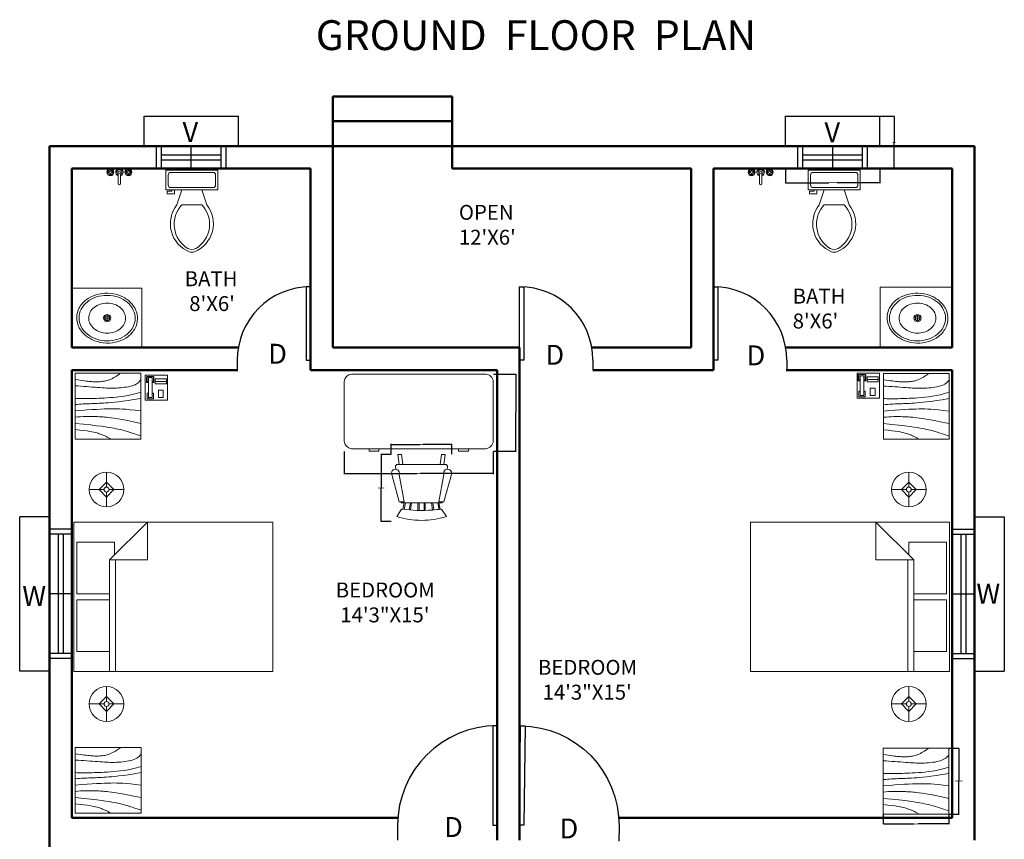
# Model space of a CAD drawing. Units: inches. Extents: x -8 to 1354, y -679 to 94.
# Tile 3 of 6: x -8 to 388, y -248 to 81. Entities that reach past the tile are written whole.
import ezdxf

# ---------------------------------------------------------------- set-up
doc = ezdxf.new("R2010")
doc.units = ezdxf.units.IN
doc.header["$MEASUREMENT"] = 0
for name, color, linetype, lineweight in [('A-ANNO-DIMS', 2, 'Continuous', 18), ('A-ANNO-TEXT', 7, 'Continuous', 25), ('A-AREA-IDEN', 7, 'Continuous', 25), ('A-DOOR', 3, 'Continuous', 25), ('A-FLOR-FIXT', 8, 'Continuous', 18), ('A-FURN', 8, 'Continuous', 18), ('A-GLAZ', 4, 'Continuous', 25), ('A-WALL', 1, 'Continuous', 50)]:
    doc.layers.add(name, color=color, linetype=linetype, lineweight=lineweight)
doc.styles.get("Standard").update_dxf_attribs({"font": 'arial.ttf'})
doc.dimstyles.get("Standard").update_dxf_attribs({"dimtxt": 0.18, "dimasz": 0.18, "dimexe": 0.18, "dimexo": 0.0625, "dimgap": 0.09, "dimtad": 0, "dimtih": 1, "dimtoh": 1, "dimdec": 1, "dimzin": 0, "dimdsep": 46, "dimlunit": 4, "dimtxsty": 'Standard', "dimcen": 0.09, "dimclrd": 2, "dimclre": 3, "dimclrt": 6, "dimadec": 0, "dimazin": 0, "dimtfac": 1, "dimtdec": 1, "dimtofl": 0, "dimtmove": 0, "dimatfit": 3, "dimfxl": 1, "dimtfill": 2, "dimtfillclr": 4, "dimtolj": 1, "dimtzin": 0, "dimarcsym": 0})

# ---------------------------------------------------------------- blocks, each defined once
blk = doc.blocks.new('*U6')
for p, q in [((0, 0), (0, -6)), ((-40, 0), (-40, -6))]:
    blk.add_line(p, q)
blk.add_lwpolyline([(0, 0), (0, 40), (-1.75, 40), (-1.75, 0)], close=True)
blk.add_arc((0, 0), 40, 90, 180)
blk = doc.blocks.new('*U4')
for p, q in [((0, 0), (0, -100)), ((750, 0), (750, -100))]:
    blk.add_line(p, q)
blk.add_lwpolyline([(0, 0), (0, 750), (43.75, 750), (43.75, 0)], close=True)
blk.add_arc((0, 0), 750, 0, 90)
blk = doc.blocks.new('*U7')
for p, q in [((-750, 0), (-750, -100)), ((0, 0), (0, -100))]:
    blk.add_line(p, q)
blk.add_lwpolyline([(0, 0), (0, 750), (-43.75, 750), (-43.75, 0)], close=True)
blk.add_arc((0, 0), 750, 90, 180)
blk = doc.blocks.new('Bed - Queen')
for p, q in [((0, -80.00003), (0, 0)), ((0, 0), (59.99999, 0)), ((59.99999, 0), (59.99999, -80.00003)), ((7.99999, -1.2), (28.79998, -1.2)), ((7.99999, -14.4), (7.99999, -1.2)), ((28.79998, -1.2), (28.79998, -14.4)), ((31.19999, -1.2), (51.99999, -1.2)), ((31.19999, -14.4), (31.19999, -1.2)), ((51.99999, -1.2), (51.99999, -16.4)), ((0, -14.4), (44.8, -14.4)), ((59.99999, -29.6), (44.8, -14.4)), ((44.8, -14.4), (44.8, -29.6)), ((44.8, -16.8), (0, -16.8)), ((51.99999, -16.4), (46.79936, -16.4)), ((44.8, -29.6), (59.99999, -29.6)), ((59.99999, -80.00003), (0, -80.00003))]:
    blk.add_line(p, q)
blk = doc.blocks.new('Chair - Rocking')
for p, q in [((-8, -4.5), (-10, -1.5)), ((8, -4.5), (10, -1.5)), ((-9, -7.5), (-12, -18.49999)), ((-7, -7.5), (-9, -7.5)), ((-9, -18.49999), (-7, -7.5)), ((-8.23428, -6.99939), (-8.3093, -7.47958)), ((-8.23041, -7), (8.23915, -7)), ((-7.5, -4.5), (-7, -7)), ((-6.5, -7), (-7.02225, -4.43)), ((-4.5, -7), (-4.96674, -4.19951)), ((-4, -7), (-4.40532, -4.16272)), ((-1.5, -4.05012), (-1.5, -7)), ((-1, -7), (-1, -4.05012)), ((1, -7), (1, -4.04655)), ((1.5, -4.05012), (1.5, -7)), ((4, -7), (4.40187, -4.18694)), ((4.5, -7), (4.96761, -4.19437)), ((6.5, -7), (7, -4.4057)), ((7.5, -4.5), (7, -7)), ((7, -7.5), (9, -7.5)), ((9, -18.49999), (7, -7.5)), ((8.31071, -7.48854), (8.23449, -7.00073)), ((9, -7.5), (12, -18.49999)), ((-10.36644, -20.64523), (-10.5, -21.49999)), ((-9, -22.49999), (-9.5, -26.49999)), ((0, -22.49999), (-9.5, -22.49999)), ((-8, -26.49999), (-7.5, -22.49999)), ((0, -22.49999), (9.5, -22.49999)), ((8, -26.49999), (7.5, -22.49999)), ((9, -22.49999), (9.5, -26.49999)), ((10.5, -21.49999), (10.3575, -20.58798)), ((-9.5, -26.49999), (-8, -26.49999)), ((9.5, -26.49999), (8, -26.49999))]:
    blk.add_line(p, q)
for centre, radius, start, end in [((0, -34.08333), 34.08333, 72.93847, 107.0615), ((0, -68.25004), 64.25, 93.92211, 97.15267), ((0, -68.25004), 64.25, 82.84733, 93.92211), ((-10.5, -18.99999), 1.58114, 161.5651, 18.43495), ((10.5, -18.99999), 1.58114, 161.5651, 18.43495), ((-9.5, -21.49999), 1, 180, 270), ((9.5, -21.49999), 1, 270, 0)]:
    blk.add_arc(centre, radius, start, end)
blk = doc.blocks.new('Desk - 30 x 60 in.')
for p, q in [((-26.999995, 0), (26.999995, 0)), ((-29.999995, -27), (-29.999995, -3)), ((29.999995, -3), (29.999995, -27)), ((26.999995, -30), (-26.999995, -30)), ((-20.000005, -30), (-20.000005, -31)), ((-20.000005, -31), (-16.000005, -31)), ((-16.000005, -31), (-16.000005, -30)), ((15.999995, -31), (15.999995, -30)), ((19.999995, -31), (15.999995, -31)), ((19.999995, -30), (19.999995, -31))]:
    blk.add_line(p, q)
for centre, start, end in [((-26.499995, -3.5), 98.1301, 171.8699), ((26.499995, -3.5), 8.130102, 81.8699), ((-26.499995, -26.5), 188.1301, 261.8699), ((26.499995, -26.5), 278.1301, 351.8699)]:
    blk.add_arc(centre, 3.535534, start, end)
blk = doc.blocks.new('Lamp - Table')
for p, q in [((0, 7), (0, 1)), ((-1, 0), (-7, 0)), ((0, 3), (-3, 0)), ((-3, 0), (0, -3)), ((3, 0), (0, 3)), ((0, -3), (3, 0)), ((1, 0), (7, 0)), ((0, -1), (0, -7))]:
    blk.add_line(p, q)
for radius in [7, 1]:
    blk.add_circle((0, 0), radius)
blk = doc.blocks.new('Phone - Desk')
for p, q in [((-4.5, -5), (-4.5, 5)), ((-4.5, 5), (4.5, 5)), ((-4, 4.5), (-4, 2)), ((-3.75, 4.5), (-3.75, 2.25)), ((-1.25, 4.5), (-3.75, 4.5)), ((-3.25, 4), (-3.25, -4)), ((-3.25, 4), (-1.75, 4)), ((-1.75, -4), (-1.75, 4)), ((-1.25, 2.25), (-1.25, 4.5)), ((-1, 2), (-1, 4.5)), ((4.5, 5), (4.5, -5)), ((-4, 2), (-3.25, 2)), ((-3.75, 2.25), (-3.25, 2.25)), ((-1.75, 2.25), (-1.25, 2.25)), ((-1.75, 2), (-1, 2)), ((4, 3.5), (-0.5, 3.5)), ((-0.5, 3.5), (-0.5, 1.5)), ((-0.5, 2.5), (4, 2.5)), ((-0.5, 1.5), (4, 1.5)), ((4, 1.5), (4, 3.5)), ((-3.75, -2.25), (-3.25, -2.25)), ((-3.75, -4.5), (-3.75, -2.25)), ((-1.75, -2.25), (-1.25, -2.25)), ((-1.25, -2.25), (-1.25, -4.5)), ((2.75, -1), (0.75, -1)), ((0.75, -1), (0.75, -4)), ((2.75, -4), (2.75, -1)), ((4.5, -5), (-4.5, -5)), ((-1.25, -4.5), (-3.75, -4.5)), ((-3.25, -4), (-1.75, -4)), ((0.75, -4), (2.75, -4))]:
    blk.add_line(p, q)
blk = doc.blocks.new('Table - Square Woodgrain 42 x 42 in.')
blk.add_line((0, -42), (42, -42))
for points in [[(0, -4), (1.704, -4.2172), (3.2358, -4.4188), (4.615, -4.604), (5.8615, -4.7721), (6.9951, -4.9224), (8.0357, -5.0541), (9.0031, -5.1667), (9.9171, -5.2594), (10.7951, -5.3316), (11.6445, -5.3836), (12.4702, -5.4157), (13.277, -5.4283), (14.0698, -5.4217), (14.8535, -5.3964), (15.6331, -5.3526), (16.4133, -5.2908), (17.1986, -5.2103), (17.9913, -5.1062), (18.793, -4.9727), (19.6056, -4.8038), (20.4307, -4.5937), (21.2701, -4.3365), (22.1256, -4.0262), (22.9989, -3.6571), (23.888, -3.2272), (24.7756, -2.7516), (25.6408, -2.2491), (26.4624, -1.7387), (27.2195, -1.2395), (27.891, -0.7703), (28.456, -0.3501), (28.8934, 0.002)], [(0, -42), (0, 0), (42, 0), (42, -42)], [(0, -8), (1.8203, -8.1001), (3.6741, -8.2149), (5.5411, -8.3408), (7.4011, -8.4741), (9.2339, -8.6112), (11.0193, -8.7484), (12.7371, -8.8821), (14.3671, -9.0086), (15.8954, -9.1246), (17.3337, -9.2278), (18.6997, -9.3159), (20.0116, -9.387), (21.2871, -9.4389), (22.5442, -9.4696), (23.8008, -9.477), (25.0749, -9.459), (26.3791, -9.4137), (27.7049, -9.3403), (29.0383, -9.2382), (30.3655, -9.1068), (31.6728, -8.9455), (32.9461, -8.7535), (34.1717, -8.5304), (35.3358, -8.2756), (36.4268, -7.9863), (37.443, -7.6521), (38.3849, -7.2603), (39.253, -6.7986), (40.048, -6.2542), (40.7705, -5.6147), (41.421, -4.8674), (42, -4)], [(42, -12), (39.1784, -12.8621), (36.4519, -13.5654), (33.8246, -14.1294), (31.3004, -14.5731), (28.8832, -14.9161), (26.577, -15.1775), (24.3858, -15.3768), (22.3136, -15.5332), (20.3622, -15.6632), (18.5254, -15.7718), (16.7947, -15.8612), (15.1618, -15.9338), (13.6183, -15.9916), (12.1558, -16.0369), (10.7659, -16.0718), (9.4403, -16.0987), (8.1703, -16.1191), (6.9461, -16.1325), (5.7577, -16.1377), (4.595, -16.1335), (3.4479, -16.1188), (2.3064, -16.0924), (1.1604, -16.0532), (0, -16)], [(42, -16), (37.6529, -16.7365), (33.8802, -17.329), (30.6179, -17.7961), (27.8015, -18.1561), (25.3668, -18.4275), (23.2497, -18.6288), (21.3859, -18.7785), (19.7111, -18.8949), (18.1693, -18.9939), (16.7375, -19.0795), (15.401, -19.1534), (14.1449, -19.217), (12.9544, -19.2717), (11.8148, -19.3191), (10.7113, -19.3606), (9.6291, -19.3976), (8.5534, -19.4323), (7.47, -19.4689), (6.3643, -19.5122), (5.222, -19.5672), (4.0288, -19.6386), (2.7703, -19.7313), (1.4321, -19.8501), (0, -20)], [(0, -24), (3.9243, -23.6805), (7.4766, -23.4138), (10.6891, -23.1954), (13.5943, -23.0205), (16.2247, -22.8847), (18.6125, -22.7832), (20.7903, -22.7116), (22.7903, -22.6651), (24.6563, -22.642), (26.4764, -22.6507), (28.35, -22.7024), (30.3766, -22.8084), (32.6555, -22.98), (35.2861, -23.2283), (38.3678, -23.5645), (42, -24)], [(42, -32), (37.392, -31.017), (33.4585, -30.2231), (30.1291, -29.5949), (27.3334, -29.109), (25.0009, -28.742), (23.0612, -28.4707), (21.4439, -28.2716), (20.0786, -28.1215), (18.8998, -28.0002), (17.8609, -27.9014), (16.9206, -27.8219), (16.0371, -27.7588), (15.1691, -27.709), (14.2748, -27.6693), (13.3128, -27.6368), (12.2415, -27.6083), (11.0295, -27.5824), (9.6867, -27.5643), (8.233, -27.5608), (6.6884, -27.5787), (5.0728, -27.6248), (3.4062, -27.7058), (1.7086, -27.8286), (0, -28)], [(0, -32), (5.4026, -32.5358), (9.9494, -33.019), (13.7424, -33.4553), (16.8834, -33.8505), (19.4743, -34.2106), (21.6171, -34.5413), (23.4136, -34.8486), (24.9657, -35.1382), (26.3614, -35.4156), (27.6332, -35.6841), (28.7995, -35.9467), (29.8788, -36.2064), (30.8897, -36.4661), (31.8507, -36.7288), (32.7802, -36.9973), (33.6968, -37.2747), (34.6175, -37.5635), (35.5531, -37.8651), (36.5128, -38.1805), (37.506, -38.5108), (38.5421, -38.8568), (39.6302, -39.2197), (40.7797, -39.6004), (42, -40)], [(0, -36), (3.0098, -36.2857), (5.5354, -36.5643), (7.6368, -36.8359), (9.374, -37.1009), (10.807, -37.3597), (11.9957, -37.6126), (13.0002, -37.8599), (13.8804, -38.102), (14.6874, -38.3393), (15.4365, -38.5729), (16.1338, -38.8041), (16.7858, -39.0341), (17.3987, -39.264), (17.9787, -39.4952), (18.5322, -39.7288), (19.0655, -39.9662), (19.5832, -40.2081), (20.0842, -40.4544), (20.5657, -40.7046), (21.0249, -40.9581), (21.459, -41.2144), (21.8653, -41.4731), (22.2409, -41.7335), (22.5831, -41.9951)]]:
    blk.add_lwpolyline(points)
blk = doc.blocks.new('Sink - Oval top')
for p, q in [((-1, 0), (1, 0)), ((0, 1), (0, -1))]:
    blk.add_line(p, q)
for points in [[(-12.23, 0.39, 0.117634), (-11.46, -3.36, 0.104469), (-8.88, -6.8, 0.090016), (-5.08, -9.07, 0.08192), (-0.32, -10.02, 0.08192), (4.49, -9.38, 0.090016), (8.42, -7.36, 0.104469), (11.22, -4.09, 0.117634), (12.23, -0.39, 0.117634), (11.46, 3.36, 0.104469), (8.88, 6.8, 0.090016), (5.08, 9.07, 0.08192), (0.32, 10.02, 0.08192), (-4.49, 9.38, 0.090016), (-8.42, 7.36, 0.104469), (-11.22, 4.09, 0.117634)], [(-11.29, 0.16, 0.118622), (-10.52, -3.25, 0.104678), (-8.07, -6.36, 0.089562), (-4.54, -8.37, 0.081185), (-0.13, -9.15, 0.081185), (4.3, -8.49, 0.089562), (7.89, -6.58, 0.104678), (10.42, -3.55, 0.118622), (11.29, -0.16, 0.118622), (10.52, 3.25, 0.104678), (8.07, 6.36, 0.089562), (4.54, 8.37, 0.081185), (0.13, 9.15, 0.081185), (-4.3, 8.49, 0.089562), (-7.89, 6.58, 0.104678), (-10.42, 3.55, 0.118622)], [(-7.42, 0.08, 0.118283), (-6.91, -2.17, 0.104607), (-5.29, -4.21, 0.089718), (-2.97, -5.53, 0.081436), (-0.07, -6.04, 0.081436), (2.84, -5.59, 0.089718), (5.2, -4.33, 0.104607), (6.86, -2.32, 0.118283), (7.42, -0.08, 0.118283), (6.91, 2.17, 0.104607), (5.29, 4.21, 0.089718), (2.97, 5.53, 0.081436), (0.07, 6.04, 0.081436), (-2.84, 5.59, 0.089718), (-5.2, 4.33, 0.104607), (-6.86, 2.32, 0.118283)]]:
    blk.add_lwpolyline(points, format="xyb", close=True)
for radius in [1.5, 1]:
    blk.add_circle((0, 0), radius)
blk = doc.blocks.new('Toilet - top')
for p, q in [((9.5, -6), (9.5, -2)), ((-10, -8.5), (-8, -8.5)), ((-10, -9.5), (-10, -8.5)), ((-7, -9.5), (-10, -9.5)), ((-8, -8.5), (-8, -8)), ((-7, -8), (-7, -9.5)), ((-4, -8), (-6, -14)), ((4, -8), (6, -14)), ((4, -14), (-4, -14))]:
    blk.add_line(p, q)
blk.add_lwpolyline([(10.5, -8), (10.5, 0), (-10.5, 0), (-10.5, -8)], close=True)
for points in [[(-9.5, -2), (-9.5, -6)], [(8.5, -1), (-8.5, -1)], [(-8.5, -7), (8.5, -7)]]:
    blk.add_lwpolyline(points)
for centre, radius, start, end in [((-8.62, -1.88), 0.884, 81.8699, 188.1301), ((8.62, -1.88), 0.884, 351.8699, 98.1301), ((-8.62, -6.12), 0.884, 171.8699, 278.1301), ((8.62, -6.12), 0.884, 261.8699, 8.1301), ((3.52, -21.58), 12.17, 141.4691, 247.9714), ((4.2, -21.82), 11.33, 136.3677, 238.9468), ((-3.52, -21.58), 12.17, 292.0284, 38.5307), ((-4.2, -21.82), 11.33, 301.053, 43.6321), ((0, -27.88), 4, 245.7318, 294.2682), ((0, -29), 4, 254.8605, 285.1395)]:
    blk.add_arc(centre, radius, start, end)
blk = doc.blocks.new('Faucet - Bathroom top')
for p, q in [((-4.107, 0.125), (-4.375, 0.125)), ((-3.75, 0.4788), (-3.75, 0.75)), ((-3.5, 0.482), (-3.5, 0.75)), ((-3.1461, 0.125), (-2.875, 0.125)), ((3.143, 0.125), (2.875, 0.125)), ((3.5, 0.4788), (3.5, 0.75)), ((3.75, 0.482), (3.75, 0.75)), ((4.1039, 0.125), (4.375, 0.125)), ((-4.1039, -0.125), (-4.375, -0.125)), ((-3.75, -0.4821), (-3.75, -0.75)), ((-3.5, -0.4789), (-3.5, -0.75)), ((-3.143, -0.125), (-2.875, -0.125)), ((-0.5, -0.8639), (-0.5, -4.5)), ((0.5, -4.5), (0.5, -0.8631)), ((3.1461, -0.125), (2.875, -0.125)), ((3.5, -0.4821), (3.5, -0.75)), ((3.75, -0.4789), (3.75, -0.75)), ((4.107, -0.125), (4.375, -0.125))]:
    blk.add_line(p, q)
for centre, radius in [((-3.625, 0), 1.375), ((-4.625, 0), 0.2795), ((-3.625, 0), 0.5), ((-3.625, 1), 0.2795), ((-2.625, 0), 0.2795), ((0, 0), 0.5), ((3.625, 0), 1.375), ((2.625, 0), 0.2795), ((3.625, 0), 0.5), ((3.625, 1), 0.2795), ((4.625, 0), 0.2795), ((-3.625, -1), 0.2795), ((3.625, -1), 0.2795)]:
    blk.add_circle(centre, radius)
for centre, radius, start, end in [((-3.625, 0), 1, 105.2407, 164.2093), ((-3.625, 0), 1, 16.44125, 74.07887), ((0, 0), 1.5, 289.6514, 250.3603), ((0, 0), 1, 300.3431, 239.7554), ((3.625, 0), 1, 106.12, 164.0884), ((3.625, 0), 1, 16.23422, 73.90469), ((-3.625, 0), 1, 196.2342, 253.9047), ((-3.625, 0), 1, 286.12, 344.0884), ((3.625, 0), 1, 196.4413, 254.0789), ((3.625, 0), 1, 285.2407, 344.2093), ((0, -4.5), 0.5, 180, 0)]:
    blk.add_arc(centre, radius, start, end)
blk = doc.blocks.new('WIN-W')
at = {"ltscale": 2}
for p, q in [((12, 62), (0, 62)), ((0, 0), (0, 62)), ((12, 57), (12, 62)), ((12, 5), (12, 0)), ((12, 0), (0, 0))]:
    blk.add_line(p, q, dxfattribs=at)
for p, q in [((21, 57), (12, 57)), ((21, 5), (12, 5))]:
    blk.add_line(p, q)
blk = doc.blocks.new('VENT-V')
for p, q in [((0, 9), (0, 21)), ((0, 21), (38, 21)), ((38, 9), (38, 21)), ((5, 9), (0, 9)), ((5, 0), (5, 9)), ((33, 0), (33, 9)), ((33, 9), (38, 9))]:
    blk.add_line(p, q)
blk = doc.blocks.new('*D83')
at = {"layer": 'A-ANNO-DIMS', "color": 3, "lineweight": -2, "transparency": 16777216}
for p, q in [((300.16, 21.11), (300.16, 15.29)), ((338.16, 21.11), (338.16, 15.29))]:
    blk.add_line(p, q, dxfattribs=at)
at = {"layer": 'A-ANNO-DIMS', "color": 2, "lineweight": -2, "transparency": 16777216}
for p, q in [((300.34, 15.47), (317.57, 15.47)), ((337.98, 15.47), (320.75, 15.47))]:
    blk.add_line(p, q, dxfattribs=at)
at = {"layer": 'A-ANNO-DIMS', "color": 2, "transparency": 16777216}
for points in [[(300.34, 15.5), (300.34, 15.44), (300.16, 15.47)], [(337.98, 15.5), (337.98, 15.44), (338.16, 15.47)]]:
    blk.add_solid(points, dxfattribs=at)
at = {"layer": 'Defpoints', "color": 0, "transparency": 16777216}
for p in [(300.16, 21.17), (338.16, 21.17), (338.16, 15.47)]:
    blk.add_point(p, dxfattribs=at)
at = {"layer": 'A-ANNO-DIMS', "color": 6, "transparency": 16777216, "insert": (319.16, 15.47), "char_height": 0.18, "attachment_point": 5, "bg_fill": 1, "box_fill_scale": 1.25, "bg_fill_color": 4, "bg_fill_transparency": 0}
blk.add_mtext('\\A1;VENTILATOR V 3\'-2" TYP.', dxfattribs=at)
blk = doc.blocks.new('*D84')
at = {"layer": 'A-ANNO-DIMS', "color": 3, "lineweight": -2, "transparency": 16777216}
for p, q in [((338.22, 42.17), (344.04, 42.17)), ((338.22, 21.17), (344.04, 21.17))]:
    blk.add_line(p, q, dxfattribs=at)
at = {"layer": 'A-ANNO-DIMS', "color": 2, "lineweight": -2, "transparency": 16777216}
for p, q in [((343.86, 41.99), (343.86, 31.86)), ((343.86, 21.35), (343.86, 31.49))]:
    blk.add_line(p, q, dxfattribs=at)
at = {"layer": 'A-ANNO-DIMS', "color": 2, "transparency": 16777216}
for points in [[(343.83, 41.99), (343.89, 41.99), (343.86, 42.17)], [(343.83, 21.35), (343.89, 21.35), (343.86, 21.17)]]:
    blk.add_solid(points, dxfattribs=at)
at = {"layer": 'Defpoints', "color": 0, "transparency": 16777216}
for p in [(338.16, 42.17), (343.86, 42.17), (338.16, 21.17)]:
    blk.add_point(p, dxfattribs=at)
at = {"layer": 'A-ANNO-DIMS', "color": 6, "transparency": 16777216, "insert": (343.86, 31.67), "char_height": 0.18, "attachment_point": 5, "bg_fill": 1, "box_fill_scale": 1.25, "bg_fill_color": 4, "bg_fill_transparency": 0}
blk.add_mtext('\\A1;1\'-9" TYP.', dxfattribs=at)
blk = doc.blocks.new('*D91')
at = {"layer": 'A-ANNO-DIMS', "color": 3, "lineweight": -2, "transparency": 16777216}
for p, q in [((365.95, -211.88), (370.03, -211.88)), ((365.95, -238.31), (370.03, -238.31))]:
    blk.add_line(p, q, dxfattribs=at)
at = {"layer": 'A-ANNO-DIMS', "color": 2, "lineweight": -2, "transparency": 16777216}
for p, q in [((369.85, -212.06), (369.85, -224.91)), ((369.85, -238.13), (369.85, -225.28))]:
    blk.add_line(p, q, dxfattribs=at)
at = {"layer": 'A-ANNO-DIMS', "color": 2, "transparency": 16777216}
for points in [[(369.82, -212.06), (369.88, -212.06), (369.85, -211.88)], [(369.82, -238.13), (369.88, -238.13), (369.85, -238.31)]]:
    blk.add_solid(points, dxfattribs=at)
at = {"layer": 'Defpoints', "color": 0, "transparency": 16777216}
for p in [(365.89, -211.88), (369.85, -211.88), (365.89, -238.31)]:
    blk.add_point(p, dxfattribs=at)
at = {"layer": 'A-ANNO-DIMS', "color": 6, "transparency": 16777216, "insert": (369.85, -225.1), "char_height": 0.18, "attachment_point": 5, "bg_fill": 1, "box_fill_scale": 1.25, "bg_fill_color": 4, "bg_fill_transparency": 0}
blk.add_mtext('\\A1;SIDE TABLE 2\'-2 1/2" TYP.', dxfattribs=at)
blk = doc.blocks.new('*D92')
at = {"layer": 'A-ANNO-DIMS', "color": 3, "lineweight": -2, "transparency": 16777216}
for p, q in [((339.46, -238.37), (339.46, -242.45)), ((365.89, -238.37), (365.89, -242.45))]:
    blk.add_line(p, q, dxfattribs=at)
at = {"layer": 'A-ANNO-DIMS', "color": 2, "lineweight": -2, "transparency": 16777216}
for p, q in [((339.64, -242.27), (351.83, -242.27)), ((365.71, -242.27), (353.53, -242.27))]:
    blk.add_line(p, q, dxfattribs=at)
at = {"layer": 'A-ANNO-DIMS', "color": 2, "transparency": 16777216}
for points in [[(339.64, -242.24), (339.64, -242.3), (339.46, -242.27)], [(365.71, -242.24), (365.71, -242.3), (365.89, -242.27)]]:
    blk.add_solid(points, dxfattribs=at)
at = {"layer": 'Defpoints', "color": 0, "transparency": 16777216}
for p in [(339.46, -238.31), (365.89, -238.31), (365.89, -242.27)]:
    blk.add_point(p, dxfattribs=at)
at = {"layer": 'A-ANNO-DIMS', "color": 6, "transparency": 16777216, "insert": (352.68, -242.27), "char_height": 0.18, "attachment_point": 5, "bg_fill": 1, "box_fill_scale": 1.25, "bg_fill_color": 4, "bg_fill_transparency": 0}
blk.add_mtext('\\A1;2\'-2 1/2" TYP.', dxfattribs=at)
blk = doc.blocks.new('*D115')
at = {"layer": 'A-ANNO-DIMS', "color": 3, "lineweight": -2, "transparency": 16777216}
for p, q in [((141.5, -93.76), (137.34, -93.76)), ((141.5, -120.76), (137.34, -120.76))]:
    blk.add_line(p, q, dxfattribs=at)
at = {"layer": 'A-ANNO-DIMS', "color": 2, "lineweight": -2, "transparency": 16777216}
for p, q in [((137.52, -93.94), (137.52, -107.08)), ((137.52, -120.58), (137.52, -107.45))]:
    blk.add_line(p, q, dxfattribs=at)
at = {"layer": 'A-ANNO-DIMS', "color": 2, "transparency": 16777216}
for points in [[(137.49, -93.94), (137.55, -93.94), (137.52, -93.76)], [(137.49, -120.58), (137.55, -120.58), (137.52, -120.76)]]:
    blk.add_solid(points, dxfattribs=at)
at = {"layer": 'Defpoints', "color": 0, "transparency": 16777216}
for p in [(141.57, -93.76), (137.52, -120.76), (141.57, -120.76)]:
    blk.add_point(p, dxfattribs=at)
at = {"layer": 'A-ANNO-DIMS', "color": 6, "transparency": 16777216, "insert": (137.52, -107.26), "char_height": 0.18, "attachment_point": 5, "bg_fill": 1, "box_fill_scale": 1.25, "bg_fill_color": 4, "bg_fill_transparency": 0}
blk.add_mtext('\\A1;ROCKING CHAIR 2\'-3"', dxfattribs=at)
blk = doc.blocks.new('*D116')
at = {"layer": 'A-ANNO-DIMS', "color": 3, "lineweight": -2, "transparency": 16777216}
for p, q in [((141.57, -93.7), (141.57, -89.53)), ((166, -93.7), (166, -89.53))]:
    blk.add_line(p, q, dxfattribs=at)
at = {"layer": 'A-ANNO-DIMS', "color": 2, "lineweight": -2, "transparency": 16777216}
for p, q in [((141.75, -89.71), (153.24, -89.71)), ((165.82, -89.71), (154.32, -89.71))]:
    blk.add_line(p, q, dxfattribs=at)
at = {"layer": 'A-ANNO-DIMS', "color": 2, "transparency": 16777216}
for points in [[(141.75, -89.68), (141.75, -89.74), (141.57, -89.71)], [(165.82, -89.68), (165.82, -89.74), (166, -89.71)]]:
    blk.add_solid(points, dxfattribs=at)
at = {"layer": 'Defpoints', "color": 0, "transparency": 16777216}
for p in [(141.57, -89.71), (141.57, -93.76), (166, -93.76)]:
    blk.add_point(p, dxfattribs=at)
at = {"layer": 'A-ANNO-DIMS', "color": 6, "transparency": 16777216, "insert": (153.78, -89.71), "char_height": 0.18, "attachment_point": 5, "bg_fill": 1, "box_fill_scale": 1.25, "bg_fill_color": 4, "bg_fill_transparency": 0}
blk.add_mtext('\\A1;2\'-0 1/2"', dxfattribs=at)
blk = doc.blocks.new('*D117')
at = {"layer": 'A-ANNO-DIMS', "color": 3, "lineweight": -2, "transparency": 16777216}
for p, q in [((122.65, -92.52), (122.65, -101.63)), ((182.65, -92.52), (182.65, -101.63))]:
    blk.add_line(p, q, dxfattribs=at)
at = {"layer": 'A-ANNO-DIMS', "color": 2, "lineweight": -2, "transparency": 16777216}
for p, q in [((122.83, -101.45), (151.95, -101.45)), ((182.47, -101.45), (153.35, -101.45))]:
    blk.add_line(p, q, dxfattribs=at)
at = {"layer": 'A-ANNO-DIMS', "color": 2, "transparency": 16777216}
for points in [[(122.83, -101.42), (122.83, -101.48), (122.65, -101.45)], [(182.47, -101.42), (182.47, -101.48), (182.65, -101.45)]]:
    blk.add_solid(points, dxfattribs=at)
at = {"layer": 'Defpoints', "color": 0, "transparency": 16777216}
for p in [(122.65, -92.45), (182.65, -92.45), (182.65, -101.45)]:
    blk.add_point(p, dxfattribs=at)
at = {"layer": 'A-ANNO-DIMS', "color": 6, "transparency": 16777216, "insert": (152.65, -101.45), "char_height": 0.18, "attachment_point": 5, "bg_fill": 1, "box_fill_scale": 1.25, "bg_fill_color": 4, "bg_fill_transparency": 0}
blk.add_mtext('\\A1;DESK 5\'-0"', dxfattribs=at)
blk = doc.blocks.new('*D118')
at = {"layer": 'A-ANNO-DIMS', "color": 3, "lineweight": -2, "transparency": 16777216}
for p, q in [((182.71, -61.45), (191.83, -61.45)), ((182.71, -92.45), (191.83, -92.45))]:
    blk.add_line(p, q, dxfattribs=at)
at = {"layer": 'A-ANNO-DIMS', "color": 2, "lineweight": -2, "transparency": 16777216}
for p, q in [((191.65, -61.63), (191.65, -76.77)), ((191.65, -92.27), (191.65, -77.13))]:
    blk.add_line(p, q, dxfattribs=at)
at = {"layer": 'A-ANNO-DIMS', "color": 2, "transparency": 16777216}
for points in [[(191.62, -61.63), (191.68, -61.63), (191.65, -61.45)], [(191.62, -92.27), (191.68, -92.27), (191.65, -92.45)]]:
    blk.add_solid(points, dxfattribs=at)
at = {"layer": 'Defpoints', "color": 0, "transparency": 16777216}
for p in [(182.65, -61.45), (191.65, -61.45), (182.65, -92.45)]:
    blk.add_point(p, dxfattribs=at)
at = {"layer": 'A-ANNO-DIMS', "color": 6, "transparency": 16777216, "insert": (191.65, -76.95), "char_height": 0.18, "attachment_point": 5, "bg_fill": 1, "box_fill_scale": 1.25, "bg_fill_color": 4, "bg_fill_transparency": 0}
blk.add_mtext('\\A1;2\'-7"', dxfattribs=at)

msp = doc.modelspace()

# ---------------------------------------------------------------- linework, layer by layer
at = {"layer": 'A-FLOR-FIXT'}
for p, q in [((13.16, -26.86), (41.24, -26.86)), ((41.24, -26.86), (41.24, -50.83)), ((367.16, -26.5), (338.23, -26.5)), ((338.23, -26.5), (338.23, -50.83))]:
    msp.add_line(p, q, dxfattribs=at)
at = {"layer": 'A-GLAZ'}
for p, q in [((42.16, 30.17), (42.16, 42.17)), ((42.16, 42.17), (80.16, 42.17)), ((80.16, 30.17), (80.16, 42.17)), ((47.16, 30.17), (42.16, 30.17)), ((47.16, 30.17), (42.16, 30.17)), ((47.16, 21.17), (47.16, 30.17)), ((49.16, 21.17), (49.16, 30.17)), ((61.16, 21.17), (61.16, 30.17)), ((73.16, 21.17), (73.16, 30.17)), ((75.16, 21.17), (75.16, 30.17)), ((75.16, 30.17), (80.16, 30.17)), ((307.16, 21.17), (307.16, 30.17)), ((319.16, 21.17), (319.16, 30.17)), ((331.16, 21.17), (331.16, 30.17)), ((49.16, 26.67), (73.16, 26.67)), ((49.16, 24.67), (73.16, 24.67)), ((307.16, 26.67), (331.16, 26.67)), ((307.16, 24.67), (331.16, 24.67)), ((13.16, -125.83), (4.16, -125.83)), ((7.66, -125.83), (7.66, -173.83)), ((9.66, -125.83), (9.66, -173.83)), ((367.16, -125.83), (376.16, -125.83)), ((370.66, -125.83), (370.66, -173.83)), ((372.66, -125.83), (372.66, -173.83)), ((13.16, -149.83), (4.16, -149.83)), ((367.16, -149.83), (376.16, -149.83)), ((13.16, -173.83), (4.16, -173.83)), ((367.16, -173.83), (376.16, -173.83))]:
    msp.add_line(p, q, dxfattribs=at)
at = {"layer": 'A-WALL'}
for p, q in [((118.16, 50.17), (166.14, 50.17)), ((118.16, 50.17), (118.16, 30.17)), ((166.14, 50.17), (166.16, 30.17)), ((118.16, 40.17), (166.14, 40.17)), ((4.16, 30.17), (118.16, 30.17)), ((4.16, -59.83), (4.16, 30.17)), ((118.16, 21.17), (118.16, 30.17)), ((118.16, 30.17), (166.14, 30.17)), ((166.14, 30.17), (271.16, 30.17)), ((166.16, 21.17), (166.16, 30.17)), ((271.16, 30.17), (376.16, 30.17)), ((376.16, 30.17), (376.16, -50.83)), ((13.16, 21.17), (109.16, 21.17)), ((13.16, -50.83), (13.16, 21.17)), ((109.16, 21.17), (109.16, -59.83)), ((118.16, 21.17), (118.16, -50.83)), ((166.14, 21.17), (262.16, 21.17)), ((262.16, 21.17), (262.16, -50.83)), ((271.16, 21.17), (271.16, -59.83)), ((271.16, 21.17), (367.16, 21.17)), ((367.16, 21.17), (367.16, -50.83)), ((376.16, 21.17), (376.16, -248.83)), ((80.07, -50.83), (13.16, -50.83)), ((193.16, -50.83), (118.16, -50.83)), ((193.16, -248.83), (193.16, -50.83)), ((262.16, -50.83), (222.25, -50.83)), ((367.16, -50.83), (300.25, -50.83)), ((4.16, -59.83), (4.16, -635.83)), ((13.16, -59.83), (13.16, -239.83)), ((79.9, -59.83), (13.16, -59.83)), ((118.16, -59.83), (109.16, -59.83)), ((184.16, -59.83), (109.16, -59.83)), ((184.16, -248.83), (184.16, -59.83)), ((271.16, -59.83), (222.69, -59.83)), ((367.16, -59.83), (300.38, -59.83)), ((367.16, -59.83), (367.16, -239.83)), ((13.16, -239.83), (144.27, -239.83)), ((193.16, -239.83), (193.25, -239.83)), ((233.11, -239.83), (367.16, -239.83))]:
    msp.add_line(p, q, dxfattribs=at)

# ---------------------------------------------------------------- block references
at = {"layer": 'A-DOOR', "xscale": 0.0393700787401575, "yscale": 0.0393700787401575, "zscale": 0.0393700787401575}
for name, p in [('*U7', (109.16, -55.89)), ('*U4', (193.16, -55.89)), ('*U4', (271.16, -55.89))]:
    msp.add_blockref(name, p, dxfattribs=at)
at = {"layer": 'A-DOOR'}
msp.add_blockref('*U6', (184.16, -242.83), dxfattribs=at)
at = {"layer": 'A-DOOR', "xscale": -1, "rotation": 359.399408492862}
msp.add_blockref('*U6', (193.22, -242.83), dxfattribs=at)
at = {"layer": 'A-FLOR-FIXT'}
for name, p in [('Faucet - Bathroom top', (32.26, 19.67)), ('Toilet - top', (61.41, 20.56)), ('Faucet - Bathroom top', (290.17, 19.67)), ('Toilet - top', (319.75, 20.56)), ('Sink - Oval top', (27.33, -38.96)), ('Sink - Oval top', (353.25, -38.96))]:
    msp.add_blockref(name, p, dxfattribs=at)
at = {"layer": 'A-FURN', "xscale": 0.6291681152010256, "yscale": 0.6291681152010256, "zscale": 0.6291681152010256}
for p in [(14.44, -61.15), (339.52, -61.22), (14.53, -211.59), (339.46, -211.89)]:
    msp.add_blockref('Table - Square Woodgrain 42 x 42 in.', p, dxfattribs=at)
at = {"layer": 'A-FURN'}
for name, p in [('Phone - Desk', (47.17, -66.88)), ('Desk - 30 x 60 in.', (152.65, -61.45)), ('Phone - Desk', (333.45, -66.11)), ('Lamp - Table', (27.08, -107.87)), ('Lamp - Table', (27.08, -194.08))]:
    msp.add_blockref(name, p, dxfattribs=at)
for name, p, rotation in [('Chair - Rocking', (153.78, -120.26), 180), ('Bed - Queen', (13.92, -180.98), 90)]:
    msp.add_blockref(name, p, dxfattribs=dict(at, rotation=rotation))
at = {"layer": 'A-FURN', "xscale": -1}
for p in [(349.76, -107.87), (349.76, -194.08)]:
    msp.add_blockref('Lamp - Table', p, dxfattribs=at)
at = {"layer": 'A-FURN', "xscale": -1, "rotation": 270}
msp.add_blockref('Bed - Queen', (366.13, -180.98), dxfattribs=at)
at = {"layer": 'A-GLAZ'}
for name, p in [('VENT-V', (300.16, 21.17)), ('WIN-W', (-7.84, -180.83))]:
    msp.add_blockref(name, p, dxfattribs=at)
at = {"layer": 'A-GLAZ', "rotation": 180}
msp.add_blockref('WIN-W', (388.16, -118.83), dxfattribs=at)

# ---------------------------------------------------------------- texts
at = {"layer": 'A-ANNO-TEXT', "attachment_point": 1}
for s, width, insert, char_height in [('GROUND  FLOOR  PLAN', 265.4598, (111.25, 80.79), 12), ('V', 71.0443, (57.66, 39.87), 8), ('V', 71.0443, (315.83, 39.75), 8), ('D', 71.0443, (92.13, -49.29), 8), ('D', 71.0443, (203.63, -49.7), 8), ('D', 71.0443, (284.51, -49.94), 8), ('W', 71.0443, (376.92, -145.75), 8), ('W', 71.0443, (-6.8, -146.62), 8), ('D', 71.0443, (162.88, -239.54), 8), ('D', 71.0443, (209.3, -240.11), 8)]:
    msp.add_mtext_dynamic_manual_height_columns(s, width=width, gutter_width=1, heights=[0], dxfattribs=dict(at, insert=insert, char_height=char_height))
at = {"layer": 'A-AREA-IDEN', "char_height": 6, "attachment_point": 1}
for s, insert in [("OPEN\\P12'X6'", (168.8, 6.56)), ("BATH\\P 8'X6'", (58.53, -20.12)), ("BATH\\P8'X6'", (303.05, -27.12)), ('BEDROOM\\P 14\'3"X15\'', (119.28, -145.26)), ('BEDROOM\\P 14\'3"X15\'', (200.64, -176.33))]:
    msp.add_mtext_dynamic_manual_height_columns(s, width=71.0443, gutter_width=1, heights=[0], dxfattribs=dict(at, insert=insert))

# ---------------------------------------------------------------- dimensions: what is measured, and where the dimension line sits
at = {"layer": 'A-ANNO-DIMS'}
for base, p1, p2, angle, text, picture, middle in [((343.86, 42.17), (338.16, 21.17), (338.16, 42.17), 90, '<> TYP.', '*D84', (343.86, 31.67)), ((137.52, -120.76), (141.57, -93.76), (141.57, -120.76), 270, 'ROCKING CHAIR <>', '*D115', (137.52, -107.26)), ((369.85, -211.88), (365.89, -238.31), (365.89, -211.88), 90, 'SIDE TABLE <> TYP.', '*D91', (369.85, -225.1))]:
    dim = msp.add_linear_dim(base=base, p1=p1, p2=p2, angle=angle, text=text, dimstyle='Standard', override={"dimdec": 1, "dimrnd": 0, "dimzin": 1, "dimlunit": 4, "dimfrac": 2}, dxfattribs=at)
    dim.commit()
    dim.dimension.update_dxf_attribs({"geometry": picture, "text_midpoint": middle})
for base, p1, p2, text, picture, middle in [((338.16, 15.47), (300.16, 21.17), (338.16, 21.17), 'VENTILATOR V <> TYP.', '*D83', (319.16, 15.47)), ((182.65, -101.45), (122.65, -92.45), (182.65, -92.45), 'DESK <>', '*D117', (152.65, -101.45)), ((365.89, -242.27), (339.46, -238.31), (365.89, -238.31), '<> TYP.', '*D92', (352.68, -242.27))]:
    dim = msp.add_linear_dim(base=base, p1=p1, p2=p2, text=text, dimstyle='Standard', override={"dimdec": 1, "dimrnd": 0, "dimzin": 1, "dimlunit": 4, "dimfrac": 2}, dxfattribs=at)
    dim.commit()
    dim.dimension.update_dxf_attribs({"geometry": picture, "text_midpoint": middle})
for base, p1, p2, angle, picture, middle in [((191.65, -61.45), (182.65, -92.45), (182.65, -61.45), 90, '*D118', (191.65, -76.95)), ((141.57, -89.71), (166, -93.76), (141.57, -93.76), 180, '*D116', (153.78, -89.71))]:
    dim = msp.add_linear_dim(base=base, p1=p1, p2=p2, angle=angle, dimstyle='Standard', override={"dimdec": 1, "dimrnd": 0, "dimzin": 1, "dimlunit": 4, "dimfrac": 2}, dxfattribs=at)
    dim.commit()
    dim.dimension.update_dxf_attribs({"geometry": picture, "text_midpoint": middle})

doc.saveas('drawing.dxf')
